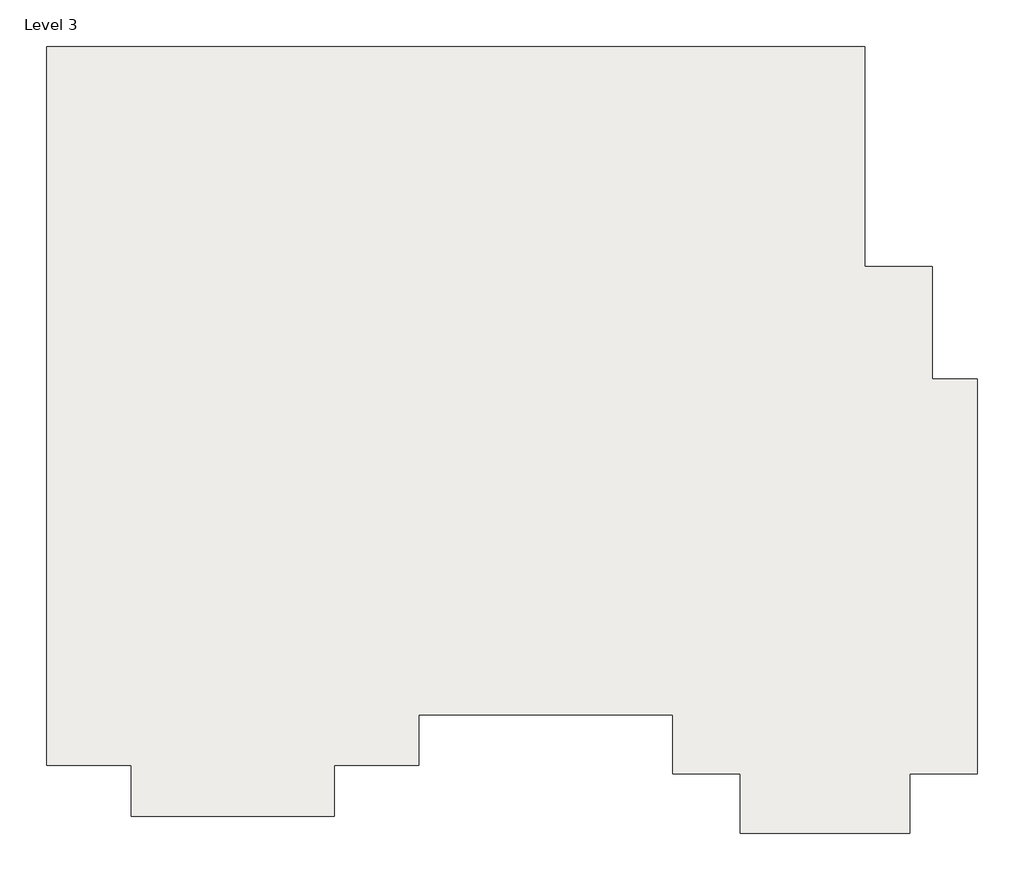
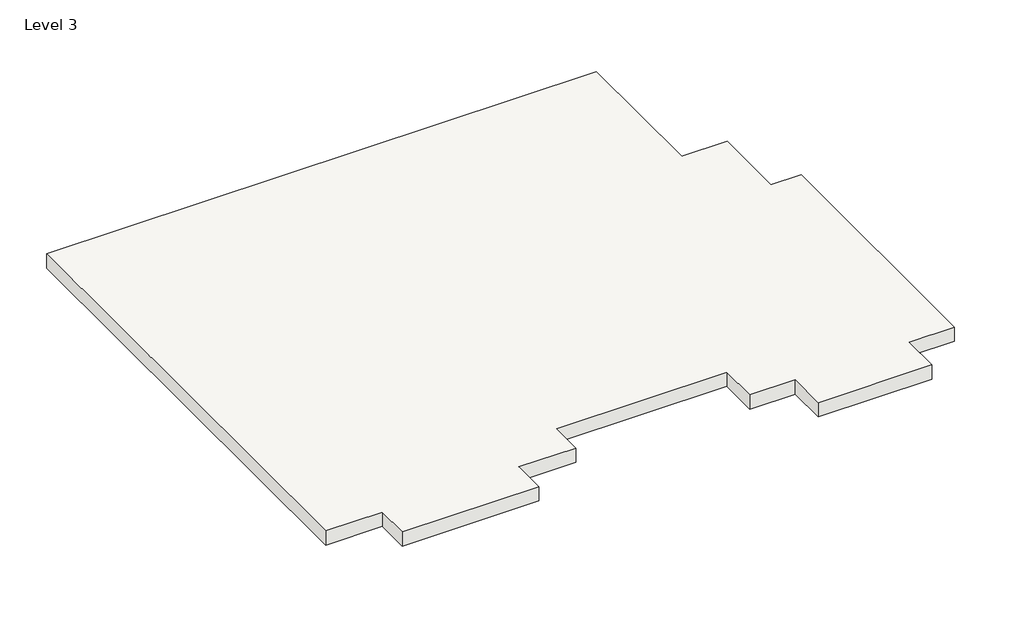
# One storey: 1 roof.
"""IFC4 building model written with IfcOpenShell, lengths in millimetres."""

from ifc_helpers import new_model, si_unit, frame, origin, place, context, project, spatial, polyline, outline, extrude, element, save

model = new_model("IFC4")

# Units and contexts
model_context = context("Model", 3, world=origin())
ifc_project = project(units=[si_unit("LENGTHUNIT", "METRE", prefix="MILLI")], contexts=[model_context])

# Site, building, storey
site = spatial("IfcSite", under=ifc_project)
building = spatial("IfcBuilding", under=site)
storey = spatial("IfcBuildingStorey", under=building, Name="Level 3", Elevation=3657.6)

# Roof
placement = place(None, origin())
element("IfcRoof", 1, ObjectType="Generic - 12\"", at=placement, inside=storey, context=model_context, shape_type="SweptSolid", body=[
    extrude(outline(polyline([(-6477.9575043, 4240.8408272), (-7620.9575043, 4240.8408272), (-7620.9575043, 13956.3408272), (3428.0424957, 13956.3408272), (3428.0424957, 10984.5408272), (4342.4424957, 10984.5408272), (4342.4424957, 9460.5408272), (4952.0424957, 9460.5408272), (4952.0424957, 4126.5408272), (4037.6424957, 4126.5408272), (4037.6424957, 3326.4408272), (1751.6424957, 3326.4408272), (1751.6424957, 4126.5408272), (837.2424957, 4126.5408272), (837.2424957, 4926.6408272), (-2591.7575043, 4926.6408272), (-2591.7575043, 4240.8408272), (-3734.7575043, 4240.8408272), (-3734.7575043, 3555.0408272), (-6477.9575043, 3555.0408272), (-6477.9575043, 4240.8408272)])), frame((0.0, 0.0, 3657.6), z_axis=(0.0, 0.0, 1.0), x_axis=(1.0, 0.0, 0.0)), (0.0, 0.0, 1.0), 304.8),
])

save(model, "model.ifc")

# Revit data of these elements
# Type "Generic - 12\""
#   Assembly Code = "B1020"
#   Layers, outside or top first: 1' - 0" no material (function 1)
# Element 1 (IfcRoof, "Generic - 12\"")
#   built-in parameter 1001705 = 13 (stored number, unit not read)
#   built-in parameter 1001710 = 33615
#   Phase Created = New Construction
#   Materials on its faces: "Default Roof"
# Materials
#   "Default Roof": colour RGB 88 101 114, transparency 0, Cost = 0
